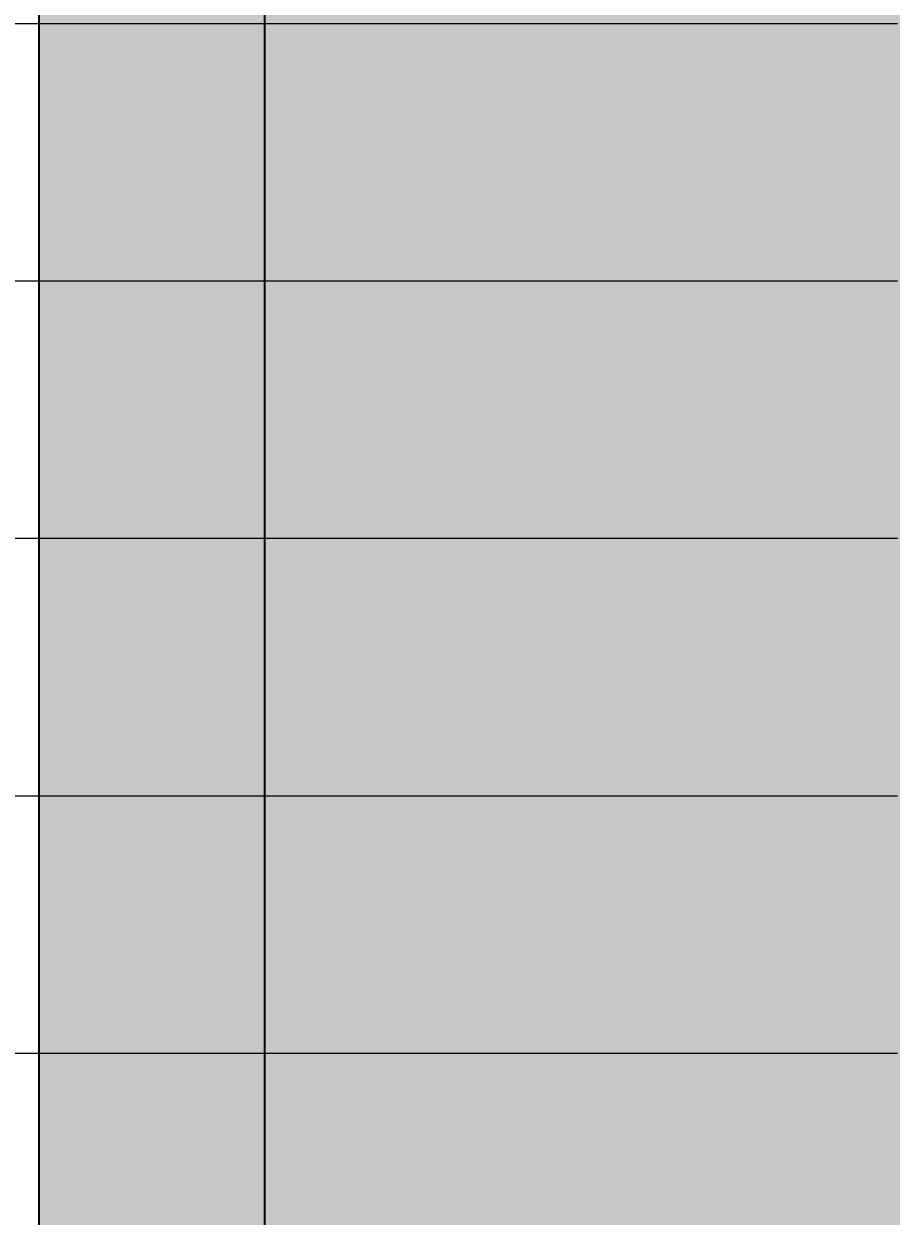
# Model space of a CAD drawing. Units: feet. Extents: x 2695 to 2912, y 795 to 1139.
# Tile 38 of 83: x 2710 to 2731, y 965 to 993. Entities that reach past the tile are written whole.
import ezdxf

# ---------------------------------------------------------------- set-up
doc = ezdxf.new("R2010")
doc.units = ezdxf.units.FT
for name, color, linetype, lineweight in [('A-ANNO-DIMS', 2, 'Continuous', 18), ('A-ELEV', 7, 'Continuous', 35), ('A-ELEV-PATT', 252, 'Continuous', 13)]:
    doc.layers.add(name, color=color, linetype=linetype, lineweight=lineweight)
doc.styles.get("Standard").update_dxf_attribs({"font": 'arial.ttf'})
doc.dimstyles.get("Standard").update_dxf_attribs({"dimtxt": 0.18, "dimasz": 0.18, "dimexe": 0.18, "dimexo": 0.0625, "dimgap": 0.09, "dimtad": 0, "dimtih": 1, "dimtoh": 1, "dimdec": 1, "dimzin": 0, "dimdsep": 46, "dimlunit": 3, "dimtxsty": 'Standard', "dimcen": 0.09, "dimadec": 0, "dimazin": 0, "dimtfac": 1, "dimtdec": 1, "dimtofl": 0, "dimtmove": 0, "dimatfit": 3, "dimfxl": 1, "dimtolj": 1, "dimtzin": 0, "dimarcsym": 0})

# ---------------------------------------------------------------- blocks, each defined once
blk = doc.blocks.new('*D12')
at = {"layer": 'A-ANNO-DIMS', "color": 0, "lineweight": -2, "transparency": 16777216}
for p, q in [((2710.574, 1122.931), (2694.681, 1122.931)), ((2694.861, 1122.751), (2694.861, 967.113)), ((2694.861, 811.111), (2694.861, 966.749)), ((2710.574, 810.931), (2694.681, 810.931))]:
    blk.add_line(p, q, dxfattribs=at)
at = {"layer": 'A-ANNO-DIMS', "color": 0, "transparency": 16777216}
for points in [[(2694.831, 1122.751), (2694.891, 1122.751), (2694.861, 1122.931)], [(2694.831, 811.111), (2694.891, 811.111), (2694.861, 810.931)]]:
    blk.add_solid(points, dxfattribs=at)
at = {"layer": 'Defpoints', "color": 0, "transparency": 16777216}
for p in [(2694.861, 1122.931), (2710.636, 1122.931), (2710.636, 810.931)]:
    blk.add_point(p, dxfattribs=at)
at = {"layer": 'A-ANNO-DIMS', "color": 0, "transparency": 16777216, "insert": (2694.861, 966.931), "char_height": 0.18, "attachment_point": 5}
blk.add_mtext('\\A1;312', dxfattribs=at)
blk = doc.blocks.new('*D32')
at = {"layer": 'A-ANNO-DIMS', "color": 0, "lineweight": -2, "transparency": 16777216}
for p, q in [((2730.646, 968.518), (2694.681, 968.518)), ((2694.861, 968.338), (2694.861, 965.7)), ((2694.861, 962.698), (2694.861, 965.336)), ((2730.646, 962.518), (2694.681, 962.518))]:
    blk.add_line(p, q, dxfattribs=at)
at = {"layer": 'A-ANNO-DIMS', "color": 0, "transparency": 16777216}
for points in [[(2694.831, 968.338), (2694.891, 968.338), (2694.861, 968.518)], [(2694.831, 962.698), (2694.891, 962.698), (2694.861, 962.518)]]:
    blk.add_solid(points, dxfattribs=at)
at = {"layer": 'Defpoints', "color": 0, "transparency": 16777216}
for p in [(2694.861, 968.518), (2730.708, 968.518), (2730.708, 962.518)]:
    blk.add_point(p, dxfattribs=at)
at = {"layer": 'A-ANNO-DIMS', "color": 0, "transparency": 16777216, "insert": (2694.861, 965.518), "char_height": 0.18, "attachment_point": 5}
blk.add_mtext('\\A1;6', dxfattribs=at)
blk = doc.blocks.new('*D33')
at = {"layer": 'A-ANNO-DIMS', "color": 0, "lineweight": -2, "transparency": 16777216}
for p, q in [((2730.646, 974.518), (2694.681, 974.518)), ((2694.861, 974.338), (2694.861, 971.7)), ((2694.861, 968.698), (2694.861, 971.336)), ((2730.646, 968.518), (2694.681, 968.518))]:
    blk.add_line(p, q, dxfattribs=at)
at = {"layer": 'A-ANNO-DIMS', "color": 0, "transparency": 16777216}
for points in [[(2694.831, 974.338), (2694.891, 974.338), (2694.861, 974.518)], [(2694.831, 968.698), (2694.891, 968.698), (2694.861, 968.518)]]:
    blk.add_solid(points, dxfattribs=at)
at = {"layer": 'Defpoints', "color": 0, "transparency": 16777216}
for p in [(2694.861, 974.518), (2730.708, 974.518), (2730.708, 968.518)]:
    blk.add_point(p, dxfattribs=at)
at = {"layer": 'A-ANNO-DIMS', "color": 0, "transparency": 16777216, "insert": (2694.861, 971.518), "char_height": 0.18, "attachment_point": 5}
blk.add_mtext('\\A1;6', dxfattribs=at)
blk = doc.blocks.new('*D34')
at = {"layer": 'A-ANNO-DIMS', "color": 0, "lineweight": -2, "transparency": 16777216}
for p, q in [((2730.646, 980.518), (2694.681, 980.518)), ((2694.861, 980.338), (2694.861, 977.7)), ((2694.861, 974.698), (2694.861, 977.336)), ((2730.646, 974.518), (2694.681, 974.518))]:
    blk.add_line(p, q, dxfattribs=at)
at = {"layer": 'A-ANNO-DIMS', "color": 0, "transparency": 16777216}
for points in [[(2694.831, 980.338), (2694.891, 980.338), (2694.861, 980.518)], [(2694.831, 974.698), (2694.891, 974.698), (2694.861, 974.518)]]:
    blk.add_solid(points, dxfattribs=at)
at = {"layer": 'Defpoints', "color": 0, "transparency": 16777216}
for p in [(2694.861, 980.518), (2730.708, 980.518), (2730.708, 974.518)]:
    blk.add_point(p, dxfattribs=at)
at = {"layer": 'A-ANNO-DIMS', "color": 0, "transparency": 16777216, "insert": (2694.861, 977.518), "char_height": 0.18, "attachment_point": 5}
blk.add_mtext('\\A1;6', dxfattribs=at)
blk = doc.blocks.new('*D35')
at = {"layer": 'A-ANNO-DIMS', "color": 0, "lineweight": -2, "transparency": 16777216}
for p, q in [((2730.646, 986.518), (2694.681, 986.518)), ((2694.861, 986.338), (2694.861, 983.7)), ((2694.861, 980.698), (2694.861, 983.336)), ((2730.646, 980.518), (2694.681, 980.518))]:
    blk.add_line(p, q, dxfattribs=at)
at = {"layer": 'A-ANNO-DIMS', "color": 0, "transparency": 16777216}
for points in [[(2694.831, 986.338), (2694.891, 986.338), (2694.861, 986.518)], [(2694.831, 980.698), (2694.891, 980.698), (2694.861, 980.518)]]:
    blk.add_solid(points, dxfattribs=at)
at = {"layer": 'Defpoints', "color": 0, "transparency": 16777216}
for p in [(2694.861, 986.518), (2730.708, 986.518), (2730.708, 980.518)]:
    blk.add_point(p, dxfattribs=at)
at = {"layer": 'A-ANNO-DIMS', "color": 0, "transparency": 16777216, "insert": (2694.861, 983.518), "char_height": 0.18, "attachment_point": 5}
blk.add_mtext('\\A1;6', dxfattribs=at)
blk = doc.blocks.new('*D36')
at = {"layer": 'A-ANNO-DIMS', "color": 0, "lineweight": -2, "transparency": 16777216}
for p, q in [((2730.646, 992.518), (2694.681, 992.518)), ((2694.861, 992.338), (2694.861, 989.7)), ((2694.861, 986.698), (2694.861, 989.336)), ((2730.646, 986.518), (2694.681, 986.518))]:
    blk.add_line(p, q, dxfattribs=at)
at = {"layer": 'A-ANNO-DIMS', "color": 0, "transparency": 16777216}
for points in [[(2694.831, 992.338), (2694.891, 992.338), (2694.861, 992.518)], [(2694.831, 986.698), (2694.891, 986.698), (2694.861, 986.518)]]:
    blk.add_solid(points, dxfattribs=at)
at = {"layer": 'Defpoints', "color": 0, "transparency": 16777216}
for p in [(2694.861, 992.518), (2730.708, 992.518), (2730.708, 986.518)]:
    blk.add_point(p, dxfattribs=at)
at = {"layer": 'A-ANNO-DIMS', "color": 0, "transparency": 16777216, "insert": (2694.861, 989.518), "char_height": 0.18, "attachment_point": 5}
blk.add_mtext('\\A1;6', dxfattribs=at)

msp = doc.modelspace()

# ---------------------------------------------------------------- hatches: boundary and pattern name
at = {"layer": 'A-ELEV-PATT'}
h = msp.add_hatch(color=256, dxfattribs=at)
h.set_gradient(color1=(255, 255, 255), tint=1)
h.paths.add_polyline_path([(2770.6361, 1122.9306), (2710.6361, 1122.9306), (2710.6361, 1118.4096), (2770.6361, 1118.4096)])
h.paths.add_polyline_path([(2890.6361, 1107.8588), (2770.6361, 1107.8588), (2770.6361, 1103.3378), (2890.6361, 1103.3378)])
h.paths.add_polyline_path([(2890.6361, 1062.9306), (2710.6361, 1062.9306), (2710.6361, 1056.9306), (2710.6361, 936.9306), (2710.6361, 924.3105), (2716.5358, 924.3105), (2890.6361, 924.3105), (2890.6361, 936.9306), (2715.8852, 936.9306), (2715.8852, 1050.3105), (2890.6361, 1050.3105)])
h.paths.add_polyline_path([(2716.5358, 924.3105), (2710.6361, 924.3105), (2710.6361, 810.9306), (2716.5358, 810.9306)])
h = msp.add_hatch(color=256, dxfattribs=at)
h.set_gradient(color1=(147, 149, 152), color2=(147, 149, 152), tint=1)
h.paths.add_polyline_path([(2770.6361, 1118.4096), (2710.6361, 1118.4096), (2710.6361, 1062.9306), (2770.6361, 1062.9306)])
h.paths.add_polyline_path([(2890.6361, 1103.3378), (2770.6361, 1103.3378), (2770.6361, 1062.9306), (2890.6361, 1062.9306)])
h.paths.add_polyline_path([(2730.7081, 1048.1052), (2755.1125, 1048.1052), (2755.1125, 936.9306), (2770.6361, 936.9306), (2770.6361, 1050.3105), (2715.8852, 1050.3105), (2715.8852, 936.9306), (2730.7081, 936.9306)])
h.paths.add_polyline_path([(2890.6361, 1050.3105), (2770.6361, 1050.3105), (2770.6361, 971.9673), (2778.0341, 971.9673), (2778.0341, 1020.8235), (2843.575, 1020.8235), (2843.575, 971.9673), (2890.6361, 971.9673)])
h.paths.add_polyline_path([(2888.1882, 970.7156), (2843.575, 970.7156), (2843.575, 964.8267), (2888.1882, 964.8267)])
h.paths.add_polyline_path([(2888.1882, 964.1328), (2843.575, 964.1328), (2843.575, 956.614), (2888.1882, 956.614)])
h.paths.add_polyline_path([(2888.1882, 955.9202), (2843.575, 955.9202), (2843.575, 949.2892), (2888.1882, 949.2892)])
h.paths.add_polyline_path([(2888.1882, 948.5954), (2843.575, 948.5954), (2843.575, 941.3507), (2888.1882, 941.3507)])
h.paths.add_polyline_path([(2888.1882, 940.6569), (2843.575, 940.6569), (2843.575, 936.9306), (2888.1882, 936.9306)])
h.paths.add_polyline_path([(2890.6361, 970.7156), (2888.9368, 970.7156), (2888.9368, 964.8267), (2890.6361, 964.8267)])
h.paths.add_polyline_path([(2890.6361, 964.1328), (2888.9368, 964.1328), (2888.9368, 956.614), (2890.6361, 956.614)])
h.paths.add_polyline_path([(2890.6361, 955.9202), (2888.9368, 955.9202), (2888.9368, 949.2892), (2890.6361, 949.2892)])
h.paths.add_polyline_path([(2890.6361, 940.6569), (2888.9368, 940.6569), (2888.9368, 936.9306), (2890.6361, 936.9306)])
h.paths.add_polyline_path([(2890.6361, 948.5954), (2888.9368, 948.5954), (2888.9368, 941.3507), (2890.6361, 941.3507)])
h.paths.add_polyline_path([(2772.5216, 970.7156), (2770.6361, 970.7156), (2770.6361, 964.8267), (2772.5216, 964.8267)])
h.paths.add_polyline_path([(2772.5216, 964.1328), (2770.6361, 964.1328), (2770.6361, 956.614), (2772.5216, 956.614)])
h.paths.add_polyline_path([(2772.5216, 955.9202), (2770.6361, 955.9202), (2770.6361, 949.2892), (2772.5216, 949.2892)])
h.paths.add_polyline_path([(2772.5216, 948.5954), (2770.6361, 948.5954), (2770.6361, 941.3507), (2772.5216, 941.3507)])
h.paths.add_polyline_path([(2772.5216, 940.6569), (2770.6361, 940.6569), (2770.6361, 936.9306), (2772.5216, 936.9306)])
h.paths.add_polyline_path([(2778.0341, 940.6569), (2773.2702, 940.6569), (2773.2702, 936.9306), (2778.0341, 936.9306)])
h.paths.add_polyline_path([(2778.0341, 970.7156), (2773.2702, 970.7156), (2773.2702, 964.8267), (2778.0341, 964.8267)])
h.paths.add_polyline_path([(2778.0341, 964.1328), (2773.2702, 964.1328), (2773.2702, 956.614), (2778.0341, 956.614)])
h.paths.add_polyline_path([(2778.0341, 955.9202), (2773.2702, 955.9202), (2773.2702, 949.2892), (2778.0341, 949.2892)])
h.paths.add_polyline_path([(2778.0341, 948.5954), (2773.2702, 948.5954), (2773.2702, 941.3507), (2778.0341, 941.3507)])
h.paths.add_polyline_path([(2810.0407, 940.6569), (2780.0341, 940.6569), (2780.0341, 936.9306), (2810.0407, 936.9306)])
h.paths.add_polyline_path([(2890.6361, 924.3105), (2770.6361, 924.3105), (2770.6361, 810.9306), (2773.5029, 810.9306), (2773.5029, 905.5143), (2805.9398, 905.5143), (2838.3767, 905.5143), (2838.3767, 810.9306), (2890.6361, 810.9306)])

# ---------------------------------------------------------------- linework, layer by layer
at = {"layer": 'A-ELEV'}
for p, q in [((2710.6361, 936.9306), (2710.6361, 1056.9306)), ((2715.8852, 1050.3105), (2715.8852, 936.9306))]:
    msp.add_line(p, q, dxfattribs=at)
msp.add_lwpolyline([(2715.8852, 1050.3105), (2715.8852, 936.9306)], dxfattribs=at)

# ---------------------------------------------------------------- dimensions: what is measured, and where the dimension line sits
at = {"layer": 'A-ANNO-DIMS'}
for base, p1, p2, picture, middle in [((2694.8611, 1122.9306), (2710.6361, 810.9306), (2710.6361, 1122.9306), '*D12', (2694.8611, 966.9306)), ((2694.8611, 992.5179), (2730.7081, 986.5179), (2730.7081, 992.5179), '*D36', (2694.8611, 989.5179)), ((2694.8611, 986.5179), (2730.7081, 980.5179), (2730.7081, 986.5179), '*D35', (2694.8611, 983.5179)), ((2694.8611, 980.5179), (2730.7081, 974.5179), (2730.7081, 980.5179), '*D34', (2694.8611, 977.5179)), ((2694.8611, 974.5179), (2730.7081, 968.5179), (2730.7081, 974.5179), '*D33', (2694.8611, 971.5179)), ((2694.8611, 968.5179), (2730.7081, 962.5179), (2730.7081, 968.5179), '*D32', (2694.8611, 965.5179))]:
    dim = msp.add_linear_dim(base=base, p1=p1, p2=p2, angle=90, dimstyle='Standard', override={"dimdec": 0, "dimlfac": 1, "dimrnd": 0, "dimzin": 0, "dimdsep": 46, "dimlunit": 2}, dxfattribs=at)
    dim.commit()
    dim.dimension.update_dxf_attribs({"geometry": picture, "text_midpoint": middle})

doc.saveas('drawing.dxf')
